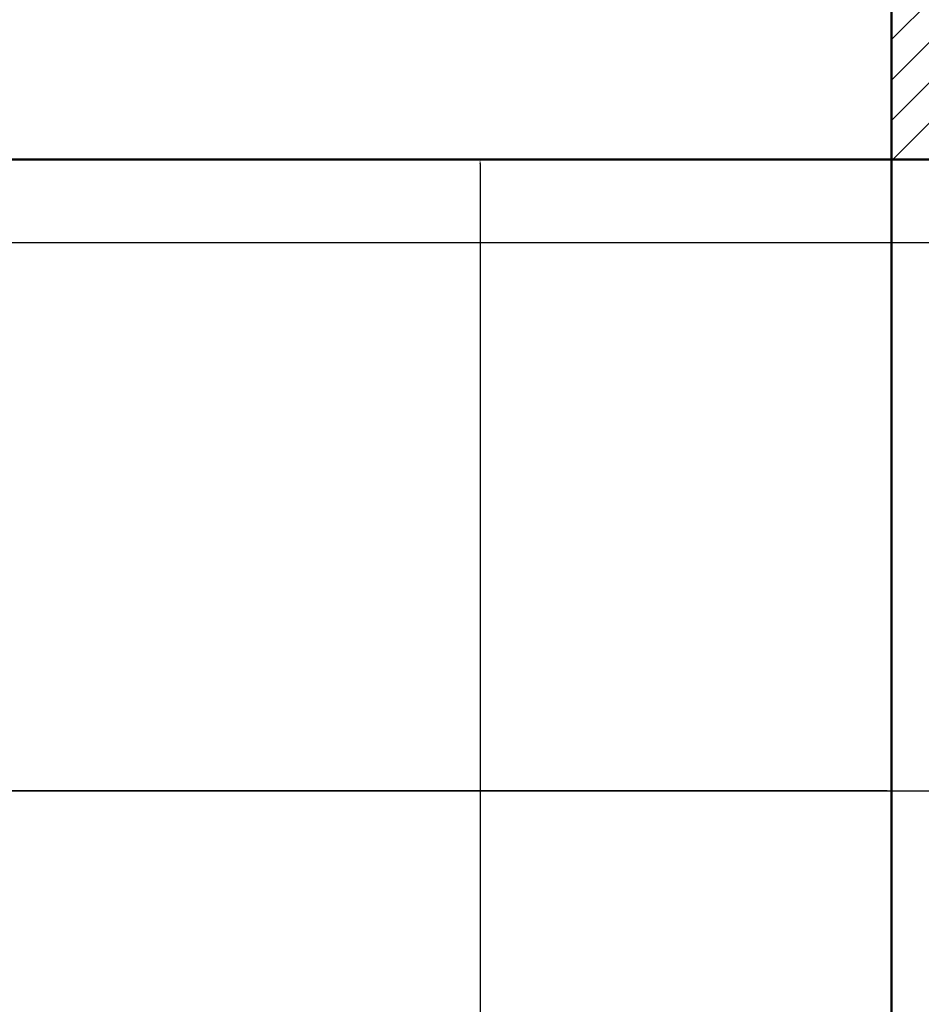
# Model space of a CAD drawing. Units: inches. Extents: x 0 to 281, y -535 to 46.
# Tile 10 of 22: x 196 to 236, y -168 to -125. Entities that reach past the tile are written whole.
import ezdxf

# ---------------------------------------------------------------- set-up
doc = ezdxf.new("R2010")
doc.units = ezdxf.units.IN
doc.header["$MEASUREMENT"] = 0
for name, color, linetype, lineweight in [('A-ANNO-DIMS', 2, 'Continuous', 18), ('A-COLS-PATT', 152, 'Continuous', 13), ('A-WALL', 7, 'Continuous', 50)]:
    doc.layers.add(name, color=color, linetype=linetype, lineweight=lineweight)
doc.styles.get("Standard").update_dxf_attribs({"font": 'arial.ttf'})
doc.dimstyles.get("Standard").update_dxf_attribs({"dimtxt": 0.18, "dimasz": 0.18, "dimexe": 0.18, "dimexo": 0.0625, "dimgap": 0.09, "dimtad": 0, "dimtih": 1, "dimtoh": 1, "dimdec": 0, "dimzin": 0, "dimdsep": 46, "dimlunit": 3, "dimtxsty": 'Standard', "dimcen": 0.09, "dimadec": 0, "dimazin": 0, "dimtfac": 1, "dimtdec": 0, "dimtofl": 0, "dimtmove": 0, "dimatfit": 3, "dimfxl": 1, "dimtolj": 1, "dimtzin": 0, "dimarcsym": 0})

# ---------------------------------------------------------------- blocks, each defined once
blk = doc.blocks.new('*D5')
at = {"layer": 'A-ANNO-DIMS', "color": 0, "lineweight": -2, "transparency": 16777216}
for p, q in [((93.459, -158.989), (93.459, -158.871)), ((93.639, -159.051), (153.846, -159.051)), ((234.279, -159.051), (174.072, -159.051)), ((234.459, -158.989), (234.459, -158.871))]:
    blk.add_line(p, q, dxfattribs=at)
at = {"layer": 'A-ANNO-DIMS', "color": 0, "transparency": 16777216}
for points in [[(93.639, -159.021), (93.639, -159.081), (93.459, -159.051)], [(234.279, -159.021), (234.279, -159.081), (234.459, -159.051)]]:
    blk.add_solid(points, dxfattribs=at)
at = {"layer": 'Defpoints', "color": 0, "transparency": 16777216}
for p in [(93.459, -159.051), (234.459, -159.051), (234.459, -159.051)]:
    blk.add_point(p, dxfattribs=at)
at = {"layer": 'A-ANNO-DIMS', "color": 0, "transparency": 16777216, "insert": (163.959, -159.051), "char_height": 6, "attachment_point": 5}
blk.add_mtext('\\A1;11\'-9"', dxfattribs=at)
blk = doc.blocks.new('*D6')
at = {"layer": 'A-ANNO-DIMS', "color": 0, "lineweight": -2, "transparency": 16777216}
for p, q in [((216.521, -131.411), (216.639, -131.411)), ((216.459, -131.591), (216.459, -194.308)), ((216.459, -263.231), (216.459, -200.513)), ((216.521, -263.411), (216.639, -263.411))]:
    blk.add_line(p, q, dxfattribs=at)
at = {"layer": 'A-ANNO-DIMS', "color": 0, "transparency": 16777216}
for points in [[(216.429, -131.591), (216.489, -131.591), (216.459, -131.411)], [(216.429, -263.231), (216.489, -263.231), (216.459, -263.411)]]:
    blk.add_solid(points, dxfattribs=at)
at = {"layer": 'Defpoints', "color": 0, "transparency": 16777216}
for p in [(216.459, -131.411), (216.459, -263.411), (216.459, -263.411)]:
    blk.add_point(p, dxfattribs=at)
at = {"layer": 'A-ANNO-DIMS', "color": 0, "transparency": 16777216, "insert": (216.459, -197.411), "char_height": 6, "attachment_point": 5}
blk.add_mtext("\\A1;11'", dxfattribs=at)
blk = doc.blocks.new('*D43')
at = {"layer": 'A-ANNO-DIMS', "color": 0, "lineweight": -2, "transparency": 16777216}
for p, q in [((93.521, -135.051), (271.089, -135.051)), ((270.909, -135.231), (270.909, -146.869)), ((270.909, -158.871), (270.909, -147.233)), ((93.521, -159.051), (271.089, -159.051))]:
    blk.add_line(p, q, dxfattribs=at)
at = {"layer": 'A-ANNO-DIMS', "color": 0, "transparency": 16777216}
for points in [[(270.879, -135.231), (270.939, -135.231), (270.909, -135.051)], [(270.879, -158.871), (270.939, -158.871), (270.909, -159.051)]]:
    blk.add_solid(points, dxfattribs=at)
at = {"layer": 'Defpoints', "color": 0, "transparency": 16777216}
for p in [(93.459, -135.051), (93.459, -159.051), (270.909, -159.051)]:
    blk.add_point(p, dxfattribs=at)
at = {"layer": 'A-ANNO-DIMS', "color": 0, "transparency": 16777216, "insert": (270.909, -147.051), "char_height": 0.18, "attachment_point": 5}
blk.add_mtext('\\A1;2\'-0"', dxfattribs=at)

msp = doc.modelspace()

# ---------------------------------------------------------------- hatches: boundary and pattern name
at = {"layer": 'A-COLS-PATT'}
h = msp.add_hatch(dxfattribs=at)
h.set_pattern_fill('ANSI31', color=256, scale=10)
h.paths.add_polyline_path([(36.459, 18.589), (27.459, 18.589), (27.459, 9.589), (36.459, 9.589)])
h.paths.add_polyline_path([(165.459, 18.589), (156.459, 18.589), (156.459, 9.589), (165.459, 9.589)])
h.paths.add_polyline_path([(243.459, 18.589), (234.459, 18.589), (234.459, 9.589), (243.459, 9.589)])
h.paths.add_polyline_path([(243.459, -122.411), (234.459, -122.411), (234.459, -131.411), (243.459, -131.411)])
h.paths.add_polyline_path([(36.459, -122.411), (27.459, -122.411), (27.459, -131.411), (36.459, -131.411)])
h.paths.add_polyline_path([(36.459, -498.411), (27.459, -498.411), (27.459, -507.411), (36.459, -507.411)])
h.paths.add_polyline_path([(243.459, -498.411), (234.459, -498.411), (234.459, -507.411), (243.459, -507.411)])
h.paths.add_polyline_path([(159.459, -498.411), (150.459, -498.411), (150.459, -507.411), (159.459, -507.411)])
h.paths.add_polyline_path([(36.459, -392.411), (27.459, -392.411), (27.459, -401.411), (36.459, -401.411)])
h.paths.add_polyline_path([(159.459, -392.411), (150.459, -392.411), (150.459, -401.411), (159.459, -401.411)])
h.paths.add_polyline_path([(243.459, -392.411), (234.459, -392.411), (234.459, -401.411), (243.459, -401.411)])
h.paths.add_polyline_path([(36.459, -263.411), (27.459, -263.411), (27.459, -272.411), (36.459, -272.411)])
h.paths.add_polyline_path([(243.459, -263.411), (234.459, -263.411), (234.459, -272.411), (243.459, -272.411)])

# ---------------------------------------------------------------- linework, layer by layer
at = {"layer": 'A-WALL'}
for p, q in [((234.459, 18.589), (234.459, -507.411)), ((189.459, -131.411), (243.459, -131.411))]:
    msp.add_line(p, q, dxfattribs=at)

# ---------------------------------------------------------------- dimensions: what is measured, and where the dimension line sits
at = {"layer": 'A-ANNO-DIMS'}
for base, p1, p2, override, picture, middle in [((216.459, -263.411), (216.459, -131.411), (216.459, -263.411), {"dimtxt": 6, "dimclrd": 0, "dimclre": 0, "dimclrt": 0}, '*D6', (216.459, -197.411)), ((270.909, -159.051), (93.459, -135.051), (93.459, -159.051), {"dimdec": 1, "dimlfac": 1, "dimrnd": 0, "dimzin": 1, "dimdsep": 46, "dimlunit": 4, "dimfrac": 2}, '*D43', (270.909, -147.051))]:
    dim = msp.add_linear_dim(base=base, p1=p1, p2=p2, angle=90, dimstyle='Standard', override=override, dxfattribs=at)
    dim.commit()
    dim.dimension.update_dxf_attribs({"geometry": picture, "text_midpoint": middle})
dim = msp.add_linear_dim(base=(234.459, -159.051), p1=(93.459, -159.051), p2=(234.459, -159.051), dimstyle='Standard', override={"dimtxt": 6, "dimclrd": 0, "dimclre": 0, "dimclrt": 0}, dxfattribs=at)
dim.commit()
dim.dimension.update_dxf_attribs({"geometry": '*D5', "text_midpoint": (163.959, -159.051)})

doc.saveas('drawing.dxf')
